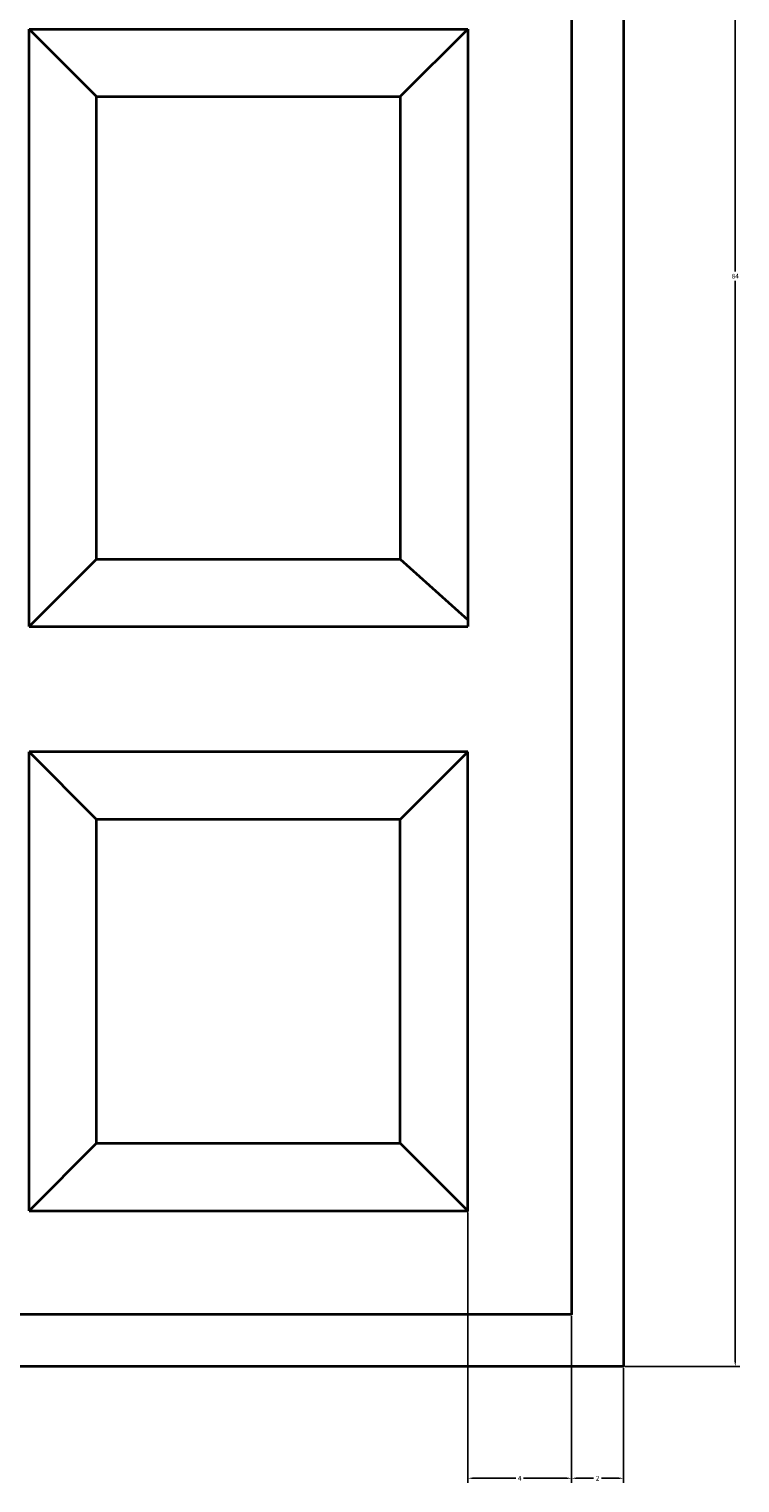
# Model space of a CAD drawing. Units: inches. Extents: x 3137 to 3299, y 1994 to 2089.
# Tile 11 of 14: x 3272 to 3299, y 1996 to 2052. Entities that reach past the tile are written whole.
import ezdxf

# ---------------------------------------------------------------- set-up
doc = ezdxf.new("R2010")
doc.units = ezdxf.units.IN
doc.header["$MEASUREMENT"] = 0
doc.layers.add('A-ANNO-DIMS', color=2, linetype='Continuous', lineweight=18)
doc.layers.add('A-DOOR', color=4, linetype='Continuous', lineweight=35)
doc.styles.get("Standard").update_dxf_attribs({"font": 'arial.ttf'})
doc.dimstyles.get("Standard").update_dxf_attribs({"dimtxt": 0.18, "dimasz": 0.18, "dimexe": 0.18, "dimexo": 0.0625, "dimgap": 0.09, "dimtad": 0, "dimtih": 1, "dimtoh": 1, "dimdec": 4, "dimzin": 0, "dimdsep": 46, "dimtxsty": 'Standard', "dimcen": 0.09, "dimadec": 0, "dimazin": 0, "dimtfac": 1, "dimtdec": 4, "dimtofl": 0, "dimtmove": 0, "dimatfit": 3, "dimfxl": 1, "dimtolj": 1, "dimtzin": 0, "dimarcsym": 0})

# ---------------------------------------------------------------- blocks, each defined once
blk = doc.blocks.new('DOOR-PANEL-RAISED-BOT')
for p, q in [((0, 17.675), (16.9, 17.675)), ((2.6, 15.075), (0, 17.675)), ((14.3, 15.075), (16.9, 17.675)), ((16.9, 0), (16.9, 17.675)), ((2.6, 15.075), (14.3, 15.075)), ((14.3, 2.6), (14.3, 15.075)), ((2.6, 2.6), (0, 0)), ((14.3, 2.6), (16.9, 0))]:
    blk.add_line(p, q)
for points in [[(16.9, 0), (0, 0), (0, 17.675)], [(14.3, 2.6), (2.6, 2.6), (2.6, 15.075)]]:
    blk.add_lwpolyline(points)
blk = doc.blocks.new('*D64')
at = {"layer": 'A-ANNO-DIMS', "color": 0, "lineweight": -2, "transparency": 16777216}
for p, q in [((3288.504, 2006.113), (3288.504, 1995.691)), ((3292.504, 2002.113), (3292.504, 1995.691)), ((3288.684, 1995.871), (3290.352, 1995.871)), ((3292.324, 1995.871), (3290.656, 1995.871))]:
    blk.add_line(p, q, dxfattribs=at)
at = {"layer": 'A-ANNO-DIMS', "color": 0, "transparency": 16777216}
for points in [[(3288.684, 1995.901), (3288.684, 1995.841), (3288.504, 1995.871)], [(3292.324, 1995.901), (3292.324, 1995.841), (3292.504, 1995.871)]]:
    blk.add_solid(points, dxfattribs=at)
at = {"layer": 'Defpoints', "color": 0, "transparency": 16777216}
for p in [(3288.504, 2006.176), (3292.504, 2002.176), (3292.504, 1995.871)]:
    blk.add_point(p, dxfattribs=at)
at = {"layer": 'A-ANNO-DIMS', "color": 0, "transparency": 16777216, "insert": (3290.504, 1995.871), "char_height": 0.18, "attachment_point": 5}
blk.add_mtext('\\A1;4', dxfattribs=at)
blk = doc.blocks.new('*D65')
at = {"layer": 'A-ANNO-DIMS', "color": 0, "lineweight": -2, "transparency": 16777216}
for p, q in [((3292.504, 2002.113), (3292.504, 1995.691)), ((3294.504, 2000.113), (3294.504, 1995.691)), ((3292.684, 1995.871), (3293.354, 1995.871)), ((3294.324, 1995.871), (3293.654, 1995.871))]:
    blk.add_line(p, q, dxfattribs=at)
at = {"layer": 'A-ANNO-DIMS', "color": 0, "transparency": 16777216}
for points in [[(3292.684, 1995.901), (3292.684, 1995.841), (3292.504, 1995.871)], [(3294.324, 1995.901), (3294.324, 1995.841), (3294.504, 1995.871)]]:
    blk.add_solid(points, dxfattribs=at)
at = {"layer": 'Defpoints', "color": 0, "transparency": 16777216}
for p in [(3292.504, 2002.176), (3294.504, 2000.176), (3294.504, 1995.871)]:
    blk.add_point(p, dxfattribs=at)
at = {"layer": 'A-ANNO-DIMS', "color": 0, "transparency": 16777216, "insert": (3293.504, 1995.871), "char_height": 0.18, "attachment_point": 5}
blk.add_mtext('\\A1;2', dxfattribs=at)
blk = doc.blocks.new('*D75')
at = {"layer": 'A-ANNO-DIMS', "color": 0, "lineweight": -2, "transparency": 16777216}
for p, q in [((3294.566, 2084.176), (3298.989, 2084.176)), ((3298.809, 2083.996), (3298.809, 2042.358)), ((3298.809, 2000.356), (3298.809, 2041.994)), ((3294.566, 2000.176), (3298.989, 2000.176))]:
    blk.add_line(p, q, dxfattribs=at)
at = {"layer": 'A-ANNO-DIMS', "color": 0, "transparency": 16777216}
for points in [[(3298.779, 2083.996), (3298.839, 2083.996), (3298.809, 2084.176)], [(3298.779, 2000.356), (3298.839, 2000.356), (3298.809, 2000.176)]]:
    blk.add_solid(points, dxfattribs=at)
at = {"layer": 'Defpoints', "color": 0, "transparency": 16777216}
for p in [(3294.504, 2084.176), (3298.809, 2084.176), (3294.504, 2000.176)]:
    blk.add_point(p, dxfattribs=at)
at = {"layer": 'A-ANNO-DIMS', "color": 0, "transparency": 16777216, "insert": (3298.809, 2042.176), "char_height": 0.18, "attachment_point": 5}
blk.add_mtext('\\A1;84', dxfattribs=at)

msp = doc.modelspace()

# ---------------------------------------------------------------- linework, layer by layer
at = {"layer": 'A-DOOR'}
for p, q in [((3271.6039, 2051.6936), (3288.5039, 2051.6936)), ((3271.6039, 2028.6759), (3271.6039, 2051.6936)), ((3274.2039, 2049.0936), (3271.6039, 2051.6936)), ((3285.9039, 2049.0936), (3288.5039, 2051.6936)), ((3274.2039, 2049.0936), (3285.9039, 2049.0936)), ((3274.2039, 2031.2759), (3274.2039, 2049.0936)), ((3274.2039, 2031.2759), (3271.6039, 2028.6759)), ((3274.2039, 2031.2759), (3285.9039, 2031.2759)), ((3285.9039, 2031.2759), (3288.5039, 2028.9346)), ((3271.6039, 2028.6759), (3288.5039, 2028.6759))]:
    msp.add_line(p, q, dxfattribs=at)
for points in [[(3234.5039, 2084.1756), (3294.5039, 2084.1756), (3294.5039, 2000.1756), (3234.5039, 2000.1756)], [(3236.5039, 2082.1756), (3292.5039, 2082.1756), (3292.5039, 2002.1756), (3236.5039, 2002.1756)]]:
    msp.add_lwpolyline(points, close=True, dxfattribs=at)
for points in [[(3288.5039, 2051.6936), (3288.5039, 2028.6759)], [(3285.9039, 2049.0936), (3285.9039, 2031.2759)]]:
    msp.add_lwpolyline(points, dxfattribs=at)

# ---------------------------------------------------------------- block references
at = {"layer": 'A-DOOR', "extrusion": (0, 0, -1), "zscale": -1}
msp.add_blockref('DOOR-PANEL-RAISED-BOT', (-3288.5039, 2006.176), dxfattribs=at)

# ---------------------------------------------------------------- dimensions: what is measured, and where the dimension line sits
at = {"layer": 'A-ANNO-DIMS'}
dim = msp.add_linear_dim(base=(3298.8089, 2084.1756), p1=(3294.5039, 2000.1756), p2=(3294.5039, 2084.1756), angle=90, dimstyle='Standard', override={"dimdec": 0, "dimlfac": 1, "dimrnd": 0, "dimzin": 0, "dimdsep": 46, "dimlunit": 2}, dxfattribs=at)
dim.commit()
dim.dimension.update_dxf_attribs({"geometry": '*D75', "text_midpoint": (3298.8089, 2042.1756)})
for base, p1, p2, picture, middle in [((3292.5039, 1995.8706), (3288.5039, 2006.1756), (3292.5039, 2002.1756), '*D64', (3290.5039, 1995.8706)), ((3294.5039, 1995.8706), (3292.5039, 2002.1756), (3294.5039, 2000.1756), '*D65', (3293.5039, 1995.8706))]:
    dim = msp.add_linear_dim(base=base, p1=p1, p2=p2, dimstyle='Standard', override={"dimdec": 0, "dimlfac": 1, "dimrnd": 0, "dimzin": 0, "dimdsep": 46, "dimlunit": 2}, dxfattribs=at)
    dim.commit()
    dim.dimension.update_dxf_attribs({"geometry": picture, "text_midpoint": middle})

doc.saveas('drawing.dxf')
